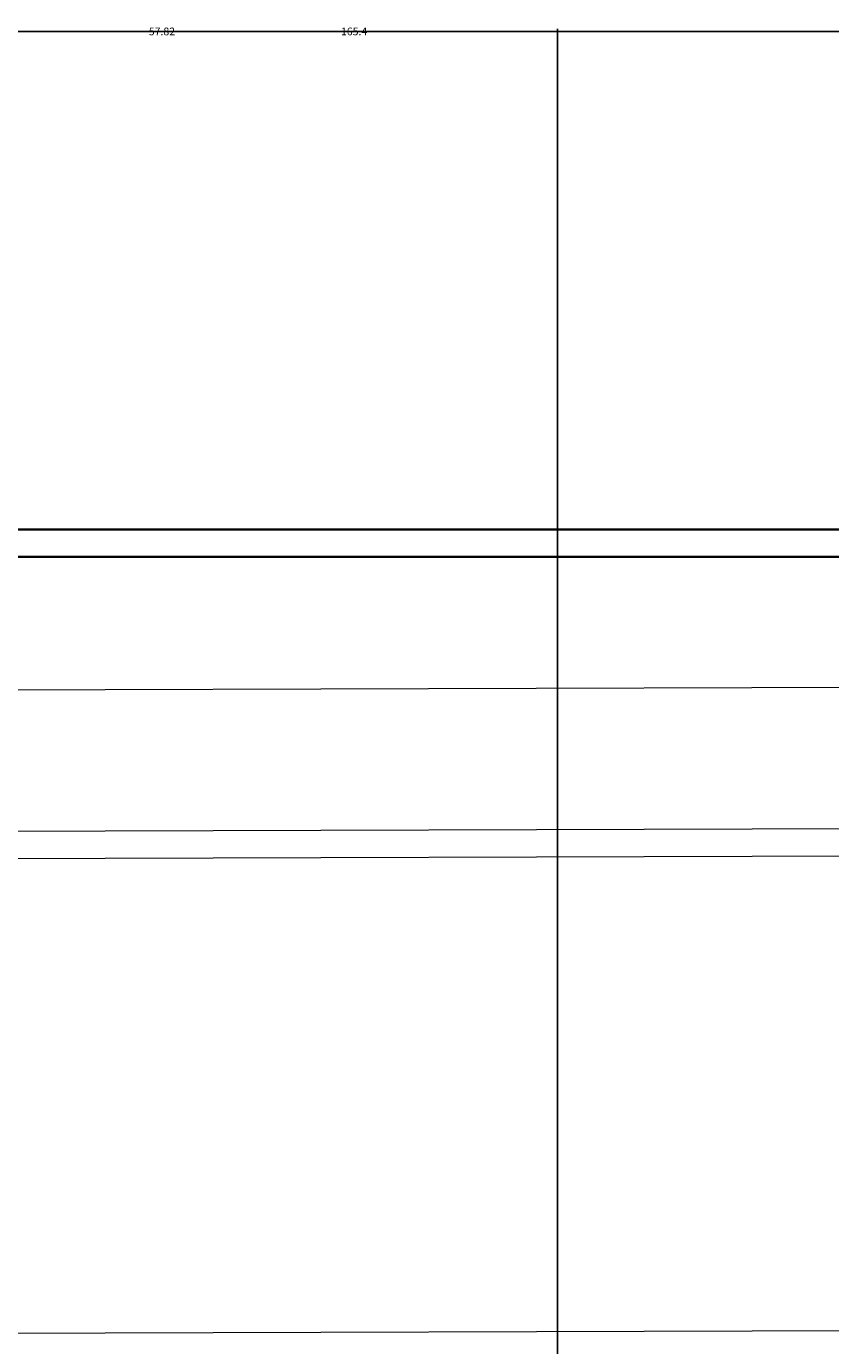
# Model space of a CAD drawing. Units: inches. Extents: x -26 to 776, y -22 to 650.
# Tile 37 of 62: x 250 to 309, y 554 to 650. Entities that reach past the tile are written whole.
import ezdxf

# ---------------------------------------------------------------- set-up
doc = ezdxf.new("R2010")
doc.units = ezdxf.units.IN
doc.header["$MEASUREMENT"] = 0
for name, color, linetype, lineweight in [('A-ANNO-DIMS', 2, 'Continuous', 18), ('A-ROOF', 7, 'Continuous', 35), ('A-WALL-TRIM', 7, 'Continuous', 18)]:
    doc.layers.add(name, color=color, linetype=linetype, lineweight=lineweight)
doc.styles.get("Standard").update_dxf_attribs({"font": 'arial.ttf'})
doc.dimstyles.get("Standard").update_dxf_attribs({"dimtxt": 0.5625, "dimasz": 0.18, "dimexe": 0.18, "dimexo": 0.0625, "dimgap": 0.09, "dimtad": 0, "dimtih": 1, "dimtoh": 1, "dimdec": 4, "dimzin": 0, "dimdsep": 46, "dimlunit": 4, "dimtxsty": 'Standard', "dimcen": 0.09, "dimadec": 0, "dimazin": 0, "dimtfac": 1, "dimtdec": 4, "dimtofl": 0, "dimtmove": 0, "dimatfit": 3, "dimfxl": 1, "dimtolj": 1, "dimtzin": 0, "dimarcsym": 0})

# ---------------------------------------------------------------- blocks, each defined once
blk = doc.blocks.new('*D16')
at = {"layer": 'A-ANNO-DIMS', "color": 0, "lineweight": -2, "transparency": 16777216}
for p, q in [((231.425, 504.483), (231.425, 649.856)), ((231.605, 649.676), (259.297, 649.676)), ((289.062, 649.676), (261.37, 649.676)), ((289.242, 504.483), (289.242, 649.856))]:
    blk.add_line(p, q, dxfattribs=at)
at = {"layer": 'A-ANNO-DIMS', "color": 0, "transparency": 16777216}
for points in [[(231.605, 649.706), (231.605, 649.646), (231.425, 649.676)], [(289.062, 649.706), (289.062, 649.646), (289.242, 649.676)]]:
    blk.add_solid(points, dxfattribs=at)
at = {"layer": 'Defpoints', "color": 0, "transparency": 16777216}
for p in [(289.242, 649.676), (231.425, 504.42), (289.242, 504.42)]:
    blk.add_point(p, dxfattribs=at)
at = {"layer": 'A-ANNO-DIMS', "color": 0, "transparency": 16777216, "insert": (260.334, 649.676), "char_height": 0.5625, "attachment_point": 5}
blk.add_mtext('\\A1;57.82', dxfattribs=at)
blk = doc.blocks.new('*D18')
at = {"layer": 'A-ANNO-DIMS', "color": 0, "lineweight": -2, "transparency": 16777216}
for p, q in [((191.678, 613.334), (191.678, 649.856)), ((191.858, 649.676), (273.361, 649.676)), ((356.887, 649.676), (275.384, 649.676)), ((357.067, 613.334), (357.067, 649.856))]:
    blk.add_line(p, q, dxfattribs=at)
at = {"layer": 'A-ANNO-DIMS', "color": 0, "transparency": 16777216}
for points in [[(191.858, 649.706), (191.858, 649.646), (191.678, 649.676)], [(356.887, 649.706), (356.887, 649.646), (357.067, 649.676)]]:
    blk.add_solid(points, dxfattribs=at)
at = {"layer": 'Defpoints', "color": 0, "transparency": 16777216}
for p in [(357.067, 649.676), (191.678, 613.271), (357.067, 613.271)]:
    blk.add_point(p, dxfattribs=at)
at = {"layer": 'A-ANNO-DIMS', "color": 0, "transparency": 16777216, "insert": (274.373, 649.676), "char_height": 0.5625, "attachment_point": 5}
blk.add_mtext('\\A1;165.4', dxfattribs=at)
blk = doc.blocks.new('*D39')
at = {"layer": 'A-ANNO-DIMS', "color": 0, "lineweight": -2, "transparency": 16777216}
for p, q in [((289.242, 15.545), (289.242, 649.856)), ((289.422, 649.676), (356.478, 649.676)), ((425.563, 649.676), (358.508, 649.676)), ((425.743, 15.545), (425.743, 649.856))]:
    blk.add_line(p, q, dxfattribs=at)
at = {"layer": 'A-ANNO-DIMS', "color": 0, "transparency": 16777216}
for points in [[(289.422, 649.706), (289.422, 649.646), (289.242, 649.676)], [(425.563, 649.706), (425.563, 649.646), (425.743, 649.676)]]:
    blk.add_solid(points, dxfattribs=at)
at = {"layer": 'Defpoints', "color": 0, "transparency": 16777216}
for p in [(425.743, 649.676), (289.242, 15.482), (425.743, 15.482)]:
    blk.add_point(p, dxfattribs=at)
at = {"layer": 'A-ANNO-DIMS', "color": 0, "transparency": 16777216, "insert": (357.493, 649.676), "char_height": 0.5625, "attachment_point": 5}
blk.add_mtext('\\A1;136.5', dxfattribs=at)

msp = doc.modelspace()

# ---------------------------------------------------------------- linework, layer by layer
at = {"layer": 'A-ROOF'}
for p, q in [((191.6782, 613.2713), (357.0669, 613.2713)), ((191.6782, 611.2713), (357.0669, 611.2713))]:
    msp.add_line(p, q, dxfattribs=at)
at = {"layer": 'A-WALL-TRIM'}
for p, q in [((191.8658, 601.3674), (357.1028, 601.8885)), ((191.6719, 591.0323), (357.2511, 591.5545)), ((191.6782, 589.0323), (357.2574, 589.5545)), ((191.6719, 554.3491), (357.2511, 554.8713))]:
    msp.add_line(p, q, dxfattribs=at)

# ---------------------------------------------------------------- dimensions: what is measured, and where the dimension line sits
at = {"layer": 'A-ANNO-DIMS'}
for base, p1, p2, override, picture, middle in [((357.0669, 649.6763), (191.6782, 613.2713), (357.0669, 613.2713), {"dimdec": 1, "dimlfac": 1, "dimrnd": 0, "dimzin": 0, "dimdsep": 46, "dimlunit": 2}, '*D18', (274.3725, 649.6763)), ((289.2424, 649.6763), (231.4249, 504.4205), (289.2424, 504.4205), {"dimdec": 2, "dimlfac": 1, "dimrnd": 0, "dimzin": 0, "dimdsep": 46, "dimlunit": 2}, '*D16', (260.3336, 649.6763)), ((425.7434, 649.6763), (289.2424, 15.4824), (425.7434, 15.4824), {"dimdec": 1, "dimlfac": 1, "dimrnd": 0, "dimzin": 0, "dimdsep": 46, "dimlunit": 2}, '*D39', (357.4929, 649.6763))]:
    dim = msp.add_linear_dim(base=base, p1=p1, p2=p2, dimstyle='Standard', override=override, dxfattribs=at)
    dim.commit()
    dim.dimension.update_dxf_attribs({"geometry": picture, "text_midpoint": middle})

doc.saveas('drawing.dxf')
